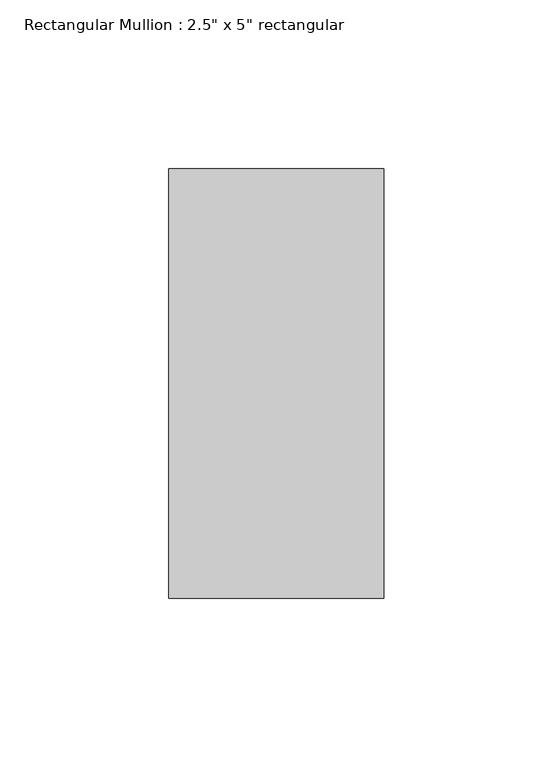
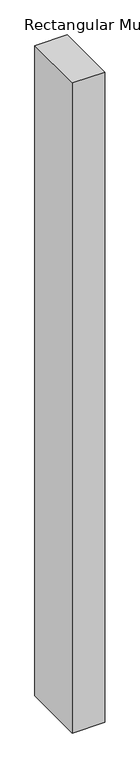
"""IFC4 building model written with IfcOpenShell, lengths in millimetres: member geometry."""

from ifc_helpers import new_model, si_unit, frame, origin, place, context, project, spatial, polyline, outline, extrude, source, transform, mapped, element, save


def member_553ffa17(model_context):
    return source(origin(), model_context, "Body", "SweptSolid", [
        extrude(outline(polyline([(31.75, 63.5), (31.75, -63.5), (-31.75, -63.5), (-31.75, 63.5), (31.75, 63.5)])), frame((0.0, 0.0, -1348.9870163), z_axis=(0.0, 0.0, 1.0), x_axis=(1.0, 0.0, 0.0)), (0.0, 0.0, 1.0), 1348.9870163),
    ])


if __name__ == "__main__":
    model = new_model("IFC4")
    model_context = context("Model", 3, world=origin())
    ifc_project = project(units=[si_unit("LENGTHUNIT", "METRE", prefix="MILLI")], contexts=[model_context])
    site = spatial("IfcSite", under=ifc_project)
    building = spatial("IfcBuilding", under=site)
    placement = place(None, origin())
    member_shape = member_553ffa17(model_context)
    element("IfcMember", 1, ObjectType="Rectangular Mullion : 2.5\" x 5\" rectangular", at=placement, inside=building, context=model_context, shape_type="MappedRepresentation", body=[
        mapped(member_shape, transform((0.0, 0.0, 0.0), x_axis=(1.0, 0.0, 0.0), y_axis=(0.0, 1.0, 0.0), z_axis=(0.0, 0.0, 1.0))),
    ])
    save(model, "model.ifc")

# Revit data of these elements
# Type "Rectangular Mullion : 2.5\" x 5\" rectangular"
#   built-in parameter 1007304 = 0.416667 (stored number, unit not read)
#   built-in parameter 1007301 = 0.104167 (stored number, unit not read)
#   built-in parameter 1007300 = 0.104167 (stored number, unit not read)
# Element 1 (IfcMember, "Rectangular Mullion : 2.5\" x 5\" rectangular")
#   Materials on its faces: "Aluminum"
# Materials
#   "Aluminum": class "Metal", colour RGB 247 247 247, transparency 0, Description = "Aluminum 6061", Cost = 0
